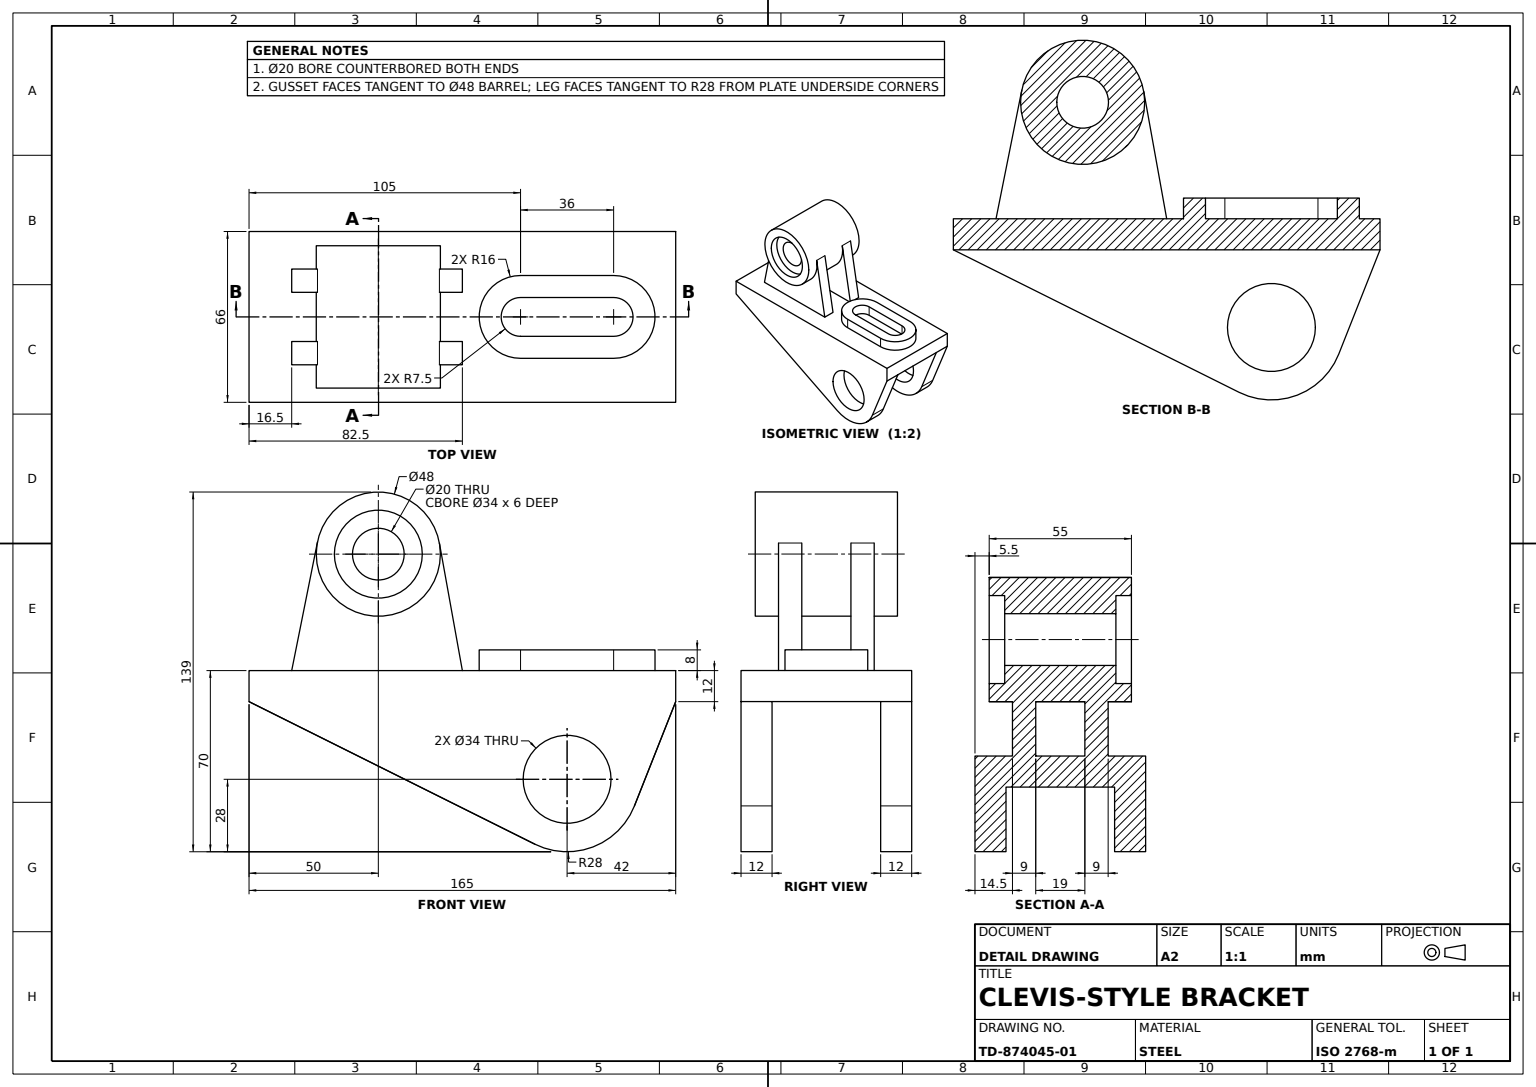
SolidWorks part; units mm, degrees
material "Plain Carbon Steel"
ref_plane "Front Plane" through (0, 0, 0) normal (0, 0, 1) x (1, 0, 0)
ref_plane "Top Plane" through (0, 0, 0) normal (0, 1, 0) x (1, 0, 0)
ref_plane "Right Plane" through (0, 0, 0) normal (1, 0, 0) x (0, 0, -1)
sketch "Stanchion Profile Sketch" plane through (0, 0, 0) normal (0, 0, 1) x (1, 0, 0)
  line L0 (0, 0) -> (165, 0)
  line L1 (0, 0) -> (0, -12)
  line L2 (0, -12) -> (110.5134, -67.0616)
  line L3 (165, 0) -> (165, -12)
  line L4 (165, -12) -> (149.0321, -52.3116)
  arc A0 (110.5134, -67.0616) -> (149.0321, -52.3116) centre (123, -42) ccw
  circle A1 centre (123, -42) radius 17
  dimension "D5" = 28
  dimension "D7" = 34
  dimension "D1" = 12
  dimension "D2" = 42
  dimension "D3" = 12
  dimension "D4" = 165
  dimension "D6" = 42
extrude "Stanchion Body" add sketch "Stanchion Profile Sketch" along normal mid plane 66
sketch "Corner Notch Sketch" plane through (165, 0, 0) normal (1, 0, 0) x (0, 0, -1)
  line L0 (-33, -12) -> (33, -12) construction
  line L1 (-21, -12) -> (21, -12)
  line L2 (-21, -12) -> (-21, -70)
  line L3 (-21, -70) -> (21, -70)
  line L4 (21, -12) -> (21, -70)
  line L5 (-33, -52.3116) -> (-33, -12) construction
  line L6 (33, -52.3116) -> (33, -12) construction
  line L7 (-33, -70) -> (33, -70) construction
  dimension "D1" = 12
  dimension "D2" = 12
extrude "Corner Notch 12x12" cut sketch "Corner Notch Sketch" against normal through all
sketch "Slotted Boss Sketch" plane through (0, 0, 0) normal (0, 1, 0) x (1, 0, 0)
  line L0 (105, 0) -> (141, 0) construction
  line L1 (105, 16) -> (141, 16)
  line L2 (105, -16) -> (141, -16)
  line L3 (105, 0) -> (141, 0) construction
  line L4 (105, 7.5) -> (141, 7.5)
  line L5 (105, -7.5) -> (141, -7.5)
  line L6 (165, -33) -> (165, 33) construction
  arc A0 (105, 16) -> (105, -16) centre (105, 0) ccw
  arc A1 (141, -16) -> (141, 16) centre (141, 0) ccw
  arc A2 (105, 7.5) -> (105, -7.5) centre (105, 0) ccw
  arc A3 (141, -7.5) -> (141, 7.5) centre (141, 0) ccw
  point P3 (123, 0)
  point P10 (123, 0)
  dimension "D2" = 16
  dimension "D1" = 15
  dimension "D3" = 42
  dimension "D4" = 36
extrude "Slotted Boss" add sketch "Slotted Boss Sketch" along normal blind 8
sketch "Hinge Barrel Sketch" plane through (0, 0, 0) normal (0, 0, 1) x (1, 0, 0)
  line L0 (165, 0) -> (0, 0) construction
  circle A0 centre (50, 45) radius 24
  circle A1 centre (50, 45) radius 10
  dimension "D1" = 48
  dimension "D2" = 20
  dimension "D3" = 45
  dimension "D4" = 50
extrude "Hinge Barrel" add sketch "Hinge Barrel Sketch" along normal mid plane 55 separate body
sketch "Barrel Gusset Sketch" plane through (0, 0, 27.5) normal (0, 0, 1) x (1, 0, 0)
  line L0 (73.6192, 49.2583) -> (82.5, 0)
  line L1 (165, 0) -> (0, 0) construction
  line L2 (26.4683, 49.718) -> (16.5, 0)
  line L3 (16.5, 0) -> (82.5, 0)
  circle A0 centre (50, 45) radius 24 construction
  arc A1 (26.4683, 49.718) -> (73.6192, 49.2583) centre (50, 45) ccw
  dimension "D1" = 66
extrude "Barrel Gusset" add sketch "Barrel Gusset Sketch" against normal blind 9 from offset 9 offset against normal yes
mirror "Barrel Gusset Mirror" about plane through (0, 0, 0) normal (0, 0, 1) of "Barrel Gusset"
sketch "Barrel Recess Sketch" plane through (0, 0, 27.5) normal (0, 0, 1) x (1, 0, 0)
  circle A0 centre (50, 45) radius 17
  dimension "D1" = 34
extrude "Barrel Recess Cut" cut sketch "Barrel Recess Sketch" against normal blind 6
mirror "Barrel Recess Mirror" about plane through (0, 0, 0) normal (0, 0, 1) of "Barrel Recess Cut"
